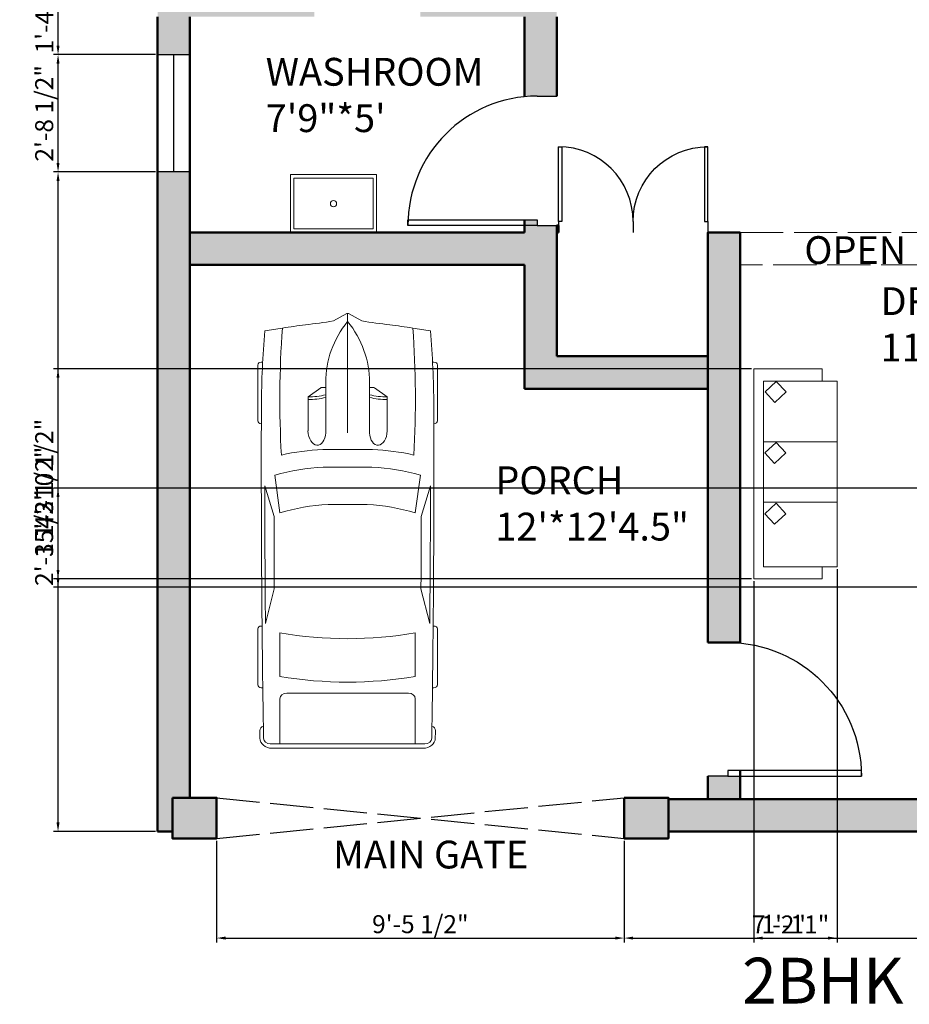
# Model space of a CAD drawing. Units: inches. Extents: x 876 to 1414, y 2665 to 3216.
# Tile 1 of 4: x 876 to 1124, y 2665 to 2939. Entities that reach past the tile are written whole.
import ezdxf

# ---------------------------------------------------------------- set-up
doc = ezdxf.new("R2010")
doc.units = ezdxf.units.IN
doc.linetypes.add('ACAD_ISO02W100', pattern=[15, 12, -3])
for name, color, linetype, lineweight in [('A-ANNO-DIMS', 2, 'Continuous', 18), ('A-ANNO-TEXT', 7, 'Continuous', 25), ('A-AREA-IDEN', 7, 'Continuous', 25), ('A-DOOR-GATE', 52, 'ACAD_ISO02W100', 25), ('A-FLOR-FIXT', 9, 'Continuous', 18), ('A-OPEN-OVHD', 210, 'ACAD_ISO02W100', 18), ('A-WALL-PATT', 252, 'Continuous', 13), ('CAR', 150, 'Continuous', 18), ('DOOR', 52, 'Continuous', 25), ('FUR', 8, 'Continuous', 18), ('WALL', 7, 'Continuous', 50), ('WIND', 130, 'Continuous', 25)]:
    doc.layers.add(name, color=color, linetype=linetype, lineweight=lineweight)
doc.styles.get("Standard").update_dxf_attribs({"font": 'arial.ttf'})
doc.dimstyles.new('ISO-25', dxfattribs={"dimtxt": 5, "dimasz": 2.5, "dimexe": 1.25, "dimexo": 0.625, "dimtad": 1, "dimdec": 0, "dimlunit": 4, "dimtxsty": 'Standard', "dimcen": 2.5, "dimadec": 0, "dimazin": 0, "dimtfac": 1, "dimtdec": 0, "dimtmove": 0, "dimatfit": 3, "dimfxl": 1, "dimarcsym": 0})

# ---------------------------------------------------------------- blocks, each defined once
blk = doc.blocks.new('*U2')
for p, q in [((0, 0), (0, -6)), ((40, 0), (40, -6))]:
    blk.add_line(p, q)
blk.add_lwpolyline([(0, 0), (0, 40), (1.75, 40), (1.75, 0)], close=True)
blk.add_arc((0, 0), 40, 0, 90)
blk = doc.blocks.new('*U4')
for p, q in [((46.55, 38.89), (22.35, 38.89)), ((136.7, 38.89), (160.9, 38.89)), ((21.1, 37.41), (21.1, 36.83)), ((47.8, 37.39), (47.8, 37.41)), ((87.99, 31.87), (74.76, 35.92)), ((134.31, 35.6), (119.29, 31.78)), ((135.45, 37.07), (135.45, 37.41)), ((162.15, 37.41), (162.15, 36.77)), ((70.03, 31.54), (86.41, 29.35)), ((186.47, -33.5), (186.47, 33.5)), ((188.4, -32.76), (188.4, 32.76)), ((138.42, 29.35), (157.25, 29.35)), ((164.52, 26.39), (164.52, -26.39)), ((186.47, 29.35), (167.01, 29.35)), ((32.27, 11.63), (36.13, 17.17)), ((36.13, 17.17), (50.94, 17.17)), ((29.77, 9.51), (51.68, 9.51)), ((32.12, 9.51), (32.12, 11.15)), ((58.92, -10.77), (58.92, 10.77)), ((66.55, -10.53), (66.55, 10.53)), ((186.47, -10.53), (186.47, 10.53)), ((3.27, 6.13), (0.1, 0.41)), ((82.74, 8.5), (82.74, -8.5)), ((0, 0), (51.68, 0)), ((0.1, -0.41), (3.27, -6.13)), ((29.77, -9.51), (51.68, -9.51)), ((32.12, -9.51), (32.12, -11.15)), ((32.27, -11.63), (36.13, -17.17)), ((36.13, -17.17), (50.94, -17.17)), ((86.41, -29.35), (70.03, -31.54)), ((157.25, -29.35), (138.42, -29.35)), ((167.01, -29.35), (186.47, -29.35)), ((87.99, -31.87), (74.76, -35.92)), ((134.31, -35.6), (119.29, -31.78)), ((21.1, -37.41), (21.1, -36.83)), ((47.8, -37.39), (47.8, -37.41)), ((135.45, -37.07), (135.45, -37.41)), ((162.15, -37.41), (162.15, -36.77)), ((46.55, -38.89), (22.35, -38.89)), ((136.7, -38.89), (160.9, -38.89))]:
    blk.add_line(p, q)
for centre, major_axis, ratio, start_param, end_param in [((22.35, 37.41), (0, -1.48), 0.842304, 3.141593, 4.712389), ((46.55, 37.41), (0, 1.48), 0.842304, -1.570796, 0), ((136.7, 37.41), (0, -1.48), 0.842304, 3.141593, 4.712389), ((160.9, 37.41), (0, 1.48), 0.842304, -1.570796, 0), ((266.03, -27.52), (0, 313.31), 0.842304, 1.367076, 1.39176), ((41.19, -490.86), (0, 528.23), 0.842304, 0.00281, 0.075598), ((64.48, -10555.62), (0, 10593.03), 0.842304, -0.013397, 0.002797), ((64.48, -10555.62), (0, -10591.55), 0.842304, 3.133765, 3.140441), ((180.63, 35.84), (0, 2.22), 0.842304, -0.013017, 1.249894), ((64.48, -10556.36), (0, 10595.31), 0.842304, -0.013397, -0.013017), ((183.98, 33.5), (0, -2.96), 0.842304, 1.570796, 3.128196), ((183.98, 32.76), (0, -5.25), 0.842304, 1.570796, 3.128196), ((135.29, 5.39), (0, 81.77), 0.842304, 1.245306, 1.50788), ((95.79, -3666.35), (0, -3698.24), 0.842304, 3.134049, 3.144098), ((259.18, -27.52), (0, -305.3), 0.842304, 4.528606, 4.561838), ((37.47, -593.96), (0, -623.33), 0.842304, 3.096046, 3.200911), ((134.4, 5.39), (0, -89.78), 0.842304, 4.449482, 4.652344), ((149.6, 2.8), (0, -79.58), 0.842304, 4.372215, 4.640744), ((17.08, 0), (0, 147.02), 0.842304, 4.511394, 4.913384), ((35.91, 0), (0, 147.02), 0.842304, 4.511394, 4.913384), ((167.01, 26.39), (0, 2.96), 0.842304, 0, 1.570796), ((-204.49, 52.4), (0, -250.96), 0.842304, 1.385369, 1.434372), ((13.04, 17.01), (0, 27.42), 0.842304, 4.435146, 4.718221), ((14.2, 17.01), (0, 27.42), 0.842304, 4.435146, 4.718221), ((50.79, 13.34), (6.34, -0.36), 0.603834, -1.395552, 1.581315), ((29.77, -46.66), (0, 56.17), 0.842304, 0, 0.590319), ((32.75, 11.15), (0, 0.74), 0.842304, 0.879714, 1.570796), ((0.62, 0), (0, -0.74), 0.842304, 4.131459, 5.293319), ((29.77, 46.66), (0, 56.17), 0.842304, 2.551274, 3.141593), ((-204.49, -52.4), (0, 250.96), 0.842304, -1.434372, -1.385369), ((149.6, -2.8), (0, -79.58), 0.842304, -1.499151, -1.230623), ((32.75, -11.15), (0, -0.74), 0.842304, 4.712389, 5.403472), ((13.04, -17.01), (0, -27.42), 0.842304, 1.564964, 1.848039), ((14.2, -17.01), (0, -27.42), 0.842304, 1.564964, 1.848039), ((134.4, -5.39), (0, -89.78), 0.842304, -1.510751, -1.307889), ((135.29, -5.39), (0, -81.77), 0.842304, -1.50788, -1.245306), ((259.18, 27.52), (0, 305.3), 0.842304, 1.721348, 1.754579), ((266.03, 27.52), (0, 313.31), 0.842304, 1.749832, 1.774517), ((37.47, 593.96), (0, -623.33), 0.842304, -0.059319, 0.045547), ((167.01, -26.39), (0, -2.96), 0.842304, 4.712389, 6.283185), ((95.79, 3666.35), (0, -3698.24), 0.842304, -0.002505, 0.007544), ((183.98, -33.5), (0, 2.96), 0.842304, 3.15499, 4.712389), ((183.98, -32.76), (0, -5.25), 0.842304, 0.013397, 1.570796), ((41.19, 490.86), (0, -528.23), 0.842304, -0.075598, -0.00281), ((22.35, -37.41), (0, 1.48), 0.842304, 1.570796, 3.141593), ((64.48, 10555.62), (0, 10593.03), 0.842304, 3.138796, 3.15499), ((46.55, -37.41), (0, -1.48), 0.842304, 0, 1.570796), ((64.48, 10555.62), (0, -10591.55), 0.842304, 0.001152, 0.007828), ((136.7, -37.41), (0, -1.48), 0.842304, -1.570796, 0), ((160.9, -37.41), (0, 1.48), 0.842304, 3.141593, 4.712389), ((180.63, -35.84), (0, -2.22), 0.842304, -1.249894, 0.013017), ((64.48, 10556.36), (0, 10595.31), 0.842304, 3.15461, 3.15499)]:
    blk.add_ellipse(centre, major_axis=major_axis, ratio=ratio, start_param=start_param, end_param=end_param)
at = {"extrusion": (0, 0, -1)}
blk.add_ellipse((50.79, -13.34), major_axis=(6.34, 0.36), ratio=0.603834, start_param=-1.395552, end_param=1.581315, dxfattribs=at)
blk = doc.blocks.new('*D31')
at = {"layer": 'A-ANNO-DIMS', "color": 0, "lineweight": -2, "transparency": 16777216}
for p, q in [((1128.58, 2808.89), (885.57, 2808.89)), ((886.82, 2783.86), (886.82, 2806.39)), ((1128.58, 2781.36), (885.57, 2781.36))]:
    blk.add_line(p, q, dxfattribs=at)
at = {"layer": 'A-ANNO-DIMS', "color": 0, "lineweight": 100, "transparency": 16777216}
for points in [[(886.4, 2806.39), (887.23, 2806.39), (886.82, 2808.89)], [(886.4, 2783.86), (887.23, 2783.86), (886.82, 2781.36)]]:
    blk.add_solid(points, dxfattribs=at)
at = {"layer": 'Defpoints', "color": 0, "lineweight": 100, "transparency": 16777216}
for p in [(886.82, 2808.89), (1129.2, 2808.89), (1129.2, 2781.36)]:
    blk.add_point(p, dxfattribs=at)
at = {"layer": 'A-ANNO-DIMS', "color": 0, "transparency": 16777216, "insert": (883.6, 2795.13), "char_height": 5, "attachment_point": 5, "rotation": 90}
blk.add_mtext('2\'-3 1/2"', dxfattribs=at)
blk = doc.blocks.new('*D32')
at = {"layer": 'A-ANNO-DIMS', "color": 0, "lineweight": -2, "transparency": 16777216}
for p, q in [((1079.71, 2842.08), (885.57, 2842.08)), ((886.82, 2786.17), (886.82, 2839.58)), ((1079.71, 2783.67), (885.57, 2783.67))]:
    blk.add_line(p, q, dxfattribs=at)
at = {"layer": 'A-ANNO-DIMS', "color": 0, "lineweight": 100, "transparency": 16777216}
for points in [[(886.4, 2839.58), (887.23, 2839.58), (886.82, 2842.08)], [(886.4, 2786.17), (887.23, 2786.17), (886.82, 2783.67)]]:
    blk.add_solid(points, dxfattribs=at)
at = {"layer": 'Defpoints', "color": 0, "lineweight": 100, "transparency": 16777216}
for p in [(886.82, 2842.08), (1080.33, 2842.08), (1080.33, 2783.67)]:
    blk.add_point(p, dxfattribs=at)
at = {"layer": 'A-ANNO-DIMS', "color": 0, "transparency": 16777216, "insert": (883.61, 2812.87), "char_height": 5, "attachment_point": 5, "rotation": 90}
blk.add_mtext('4\'-10 1/2"', dxfattribs=at)
blk = doc.blocks.new('*D33')
at = {"layer": 'A-ANNO-DIMS', "color": 0, "lineweight": -2, "transparency": 16777216}
for p, q in [((1103.5, 2786.39), (1103.5, 2682.56)), ((1080.33, 2783.04), (1080.33, 2682.56)), ((1082.83, 2683.81), (1101, 2683.81))]:
    blk.add_line(p, q, dxfattribs=at)
at = {"layer": 'A-ANNO-DIMS', "color": 0, "lineweight": 100, "transparency": 16777216}
for points in [[(1082.83, 2684.22), (1082.83, 2683.39), (1080.33, 2683.81)], [(1101, 2684.22), (1101, 2683.39), (1103.5, 2683.81)]]:
    blk.add_solid(points, dxfattribs=at)
at = {"layer": 'Defpoints', "color": 0, "lineweight": 100, "transparency": 16777216}
for p in [(1103.5, 2787.02), (1080.33, 2783.67), (1103.5, 2683.81)]:
    blk.add_point(p, dxfattribs=at)
at = {"layer": 'A-ANNO-DIMS', "color": 0, "transparency": 16777216, "insert": (1091.91, 2686.94), "char_height": 5, "attachment_point": 5}
blk.add_mtext('1\'-11"', dxfattribs=at)
blk = doc.blocks.new('*D41')
at = {"layer": 'A-ANNO-DIMS', "color": 0, "lineweight": -2, "transparency": 16777216}
for p, q in [((930.9, 2710.88), (930.9, 2682.56)), ((1044.28, 2710.88), (1044.28, 2682.56)), ((933.4, 2683.81), (1041.78, 2683.81))]:
    blk.add_line(p, q, dxfattribs=at)
at = {"layer": 'A-ANNO-DIMS', "color": 0, "lineweight": 100, "transparency": 16777216}
for points in [[(933.4, 2684.22), (933.4, 2683.39), (930.9, 2683.81)], [(1041.78, 2684.22), (1041.78, 2683.39), (1044.28, 2683.81)]]:
    blk.add_solid(points, dxfattribs=at)
at = {"layer": 'Defpoints', "color": 0, "lineweight": 100, "transparency": 16777216}
for p in [(930.9, 2711.51), (1044.28, 2711.51), (1044.28, 2683.81)]:
    blk.add_point(p, dxfattribs=at)
at = {"layer": 'A-ANNO-DIMS', "color": 0, "transparency": 16777216, "insert": (987.59, 2687.02), "char_height": 5, "attachment_point": 5}
blk.add_mtext('9\'-5 1/2"', dxfattribs=at)
blk = doc.blocks.new('*D42')
at = {"layer": 'A-ANNO-DIMS', "color": 0, "lineweight": -2, "transparency": 16777216}
for p, q in [((1130.38, 2712.82), (1130.38, 2682.56)), ((1044.28, 2710.88), (1044.28, 2682.56)), ((1046.78, 2683.81), (1127.88, 2683.81))]:
    blk.add_line(p, q, dxfattribs=at)
at = {"layer": 'A-ANNO-DIMS', "color": 0, "lineweight": 100, "transparency": 16777216}
for points in [[(1046.78, 2684.22), (1046.78, 2683.39), (1044.28, 2683.81)], [(1127.88, 2684.22), (1127.88, 2683.39), (1130.38, 2683.81)]]:
    blk.add_solid(points, dxfattribs=at)
at = {"layer": 'Defpoints', "color": 0, "lineweight": 100, "transparency": 16777216}
for p in [(1130.38, 2713.44), (1044.28, 2711.51), (1130.38, 2683.81)]:
    blk.add_point(p, dxfattribs=at)
at = {"layer": 'A-ANNO-DIMS', "color": 0, "transparency": 16777216, "insert": (1087.33, 2686.94), "char_height": 5, "attachment_point": 5}
blk.add_mtext('7\'-2"', dxfattribs=at)
blk = doc.blocks.new('*D51')
at = {"layer": 'A-ANNO-DIMS', "color": 0, "lineweight": -2, "transparency": 16777216}
for p, q in [((913.89, 2945.19), (885.57, 2945.19)), ((886.82, 2931.91), (886.82, 2942.69)), ((913.89, 2929.41), (885.57, 2929.41))]:
    blk.add_line(p, q, dxfattribs=at)
at = {"layer": 'A-ANNO-DIMS', "color": 0, "lineweight": 100, "transparency": 16777216}
for points in [[(886.4, 2942.69), (887.23, 2942.69), (886.82, 2945.19)], [(886.4, 2931.91), (887.23, 2931.91), (886.82, 2929.41)]]:
    blk.add_solid(points, dxfattribs=at)
at = {"layer": 'Defpoints', "color": 0, "lineweight": 100, "transparency": 16777216}
for p in [(886.82, 2945.19), (914.52, 2945.19), (914.52, 2929.41)]:
    blk.add_point(p, dxfattribs=at)
at = {"layer": 'A-ANNO-DIMS', "color": 0, "transparency": 16777216, "insert": (883.68, 2937.3), "char_height": 5, "attachment_point": 5, "rotation": 90}
blk.add_mtext('1\'-4"', dxfattribs=at)
blk = doc.blocks.new('*D52')
at = {"layer": 'A-ANNO-DIMS', "color": 0, "lineweight": -2, "transparency": 16777216}
for p, q in [((913.89, 2929.41), (885.57, 2929.41)), ((886.82, 2899.3), (886.82, 2926.91)), ((913.89, 2896.8), (885.57, 2896.8))]:
    blk.add_line(p, q, dxfattribs=at)
at = {"layer": 'A-ANNO-DIMS', "color": 0, "lineweight": 100, "transparency": 16777216}
for points in [[(886.4, 2926.91), (887.23, 2926.91), (886.82, 2929.41)], [(886.4, 2899.3), (887.23, 2899.3), (886.82, 2896.8)]]:
    blk.add_solid(points, dxfattribs=at)
at = {"layer": 'Defpoints', "color": 0, "lineweight": 100, "transparency": 16777216}
for p in [(886.82, 2929.41), (914.52, 2929.41), (914.52, 2896.8)]:
    blk.add_point(p, dxfattribs=at)
at = {"layer": 'A-ANNO-DIMS', "color": 0, "transparency": 16777216, "insert": (883.61, 2913.1), "char_height": 5, "attachment_point": 5, "rotation": 90}
blk.add_mtext('2\'-8 1/2"', dxfattribs=at)
blk = doc.blocks.new('*D53')
at = {"layer": 'A-ANNO-DIMS', "color": 0, "lineweight": -2, "transparency": 16777216}
for p, q in [((913.89, 2896.8), (885.57, 2896.8)), ((886.82, 2715.94), (886.82, 2894.3)), ((913.89, 2713.44), (885.57, 2713.44))]:
    blk.add_line(p, q, dxfattribs=at)
at = {"layer": 'A-ANNO-DIMS', "color": 0, "lineweight": 100, "transparency": 16777216}
for points in [[(886.4, 2894.3), (887.23, 2894.3), (886.82, 2896.8)], [(886.4, 2715.94), (887.23, 2715.94), (886.82, 2713.44)]]:
    blk.add_solid(points, dxfattribs=at)
at = {"layer": 'Defpoints', "color": 0, "lineweight": 100, "transparency": 16777216}
for p in [(886.82, 2896.8), (914.52, 2896.8), (914.52, 2713.44)]:
    blk.add_point(p, dxfattribs=at)
at = {"layer": 'A-ANNO-DIMS', "color": 0, "transparency": 16777216, "insert": (883.6, 2805.12), "char_height": 5, "attachment_point": 5, "rotation": 90}
blk.add_mtext('15\'-3 1/2"', dxfattribs=at)

msp = doc.modelspace()

# ---------------------------------------------------------------- hatches: boundary and pattern name
at = {"layer": 'A-WALL-PATT'}
h = msp.add_hatch(color=256, dxfattribs=at)
h.dxf.hatch_style = 1
h.paths.add_polyline_path([(966.14, 3166.44), (914.52, 3166.44), (914.52, 3077.43), (923.52, 3077.43), (923.52, 3157.44), (966.14, 3157.44)])
h.paths.add_polyline_path([(1117.41, 3166.44), (1072.02, 3166.44), (1025.39, 3166.44), (1025.39, 3157.44), (1067.52, 3157.44), (1067.52, 3050.33), (1068, 3050.33), (1068, 3010.33), (1068, 3004.44), (1072.02, 3004.44), (1076.39, 3004.44), (1076.39, 3010.44), (1076.39, 3013.44), (1072.02, 3013.44), (1072.02, 3157.44), (1090.31, 3157.44), (1117.41, 3157.44)])
h.paths.add_polyline_path([(1257.93, 3166.44), (1225.02, 3166.44), (1176.66, 3166.44), (1176.66, 3157.44), (1216.02, 3157.44), (1216.02, 3013.44), (1116.28, 3013.44, -0.01877), (1116.39, 3010.44), (1116.39, 3004.44), (1225.02, 3004.44), (1225.02, 3014.27), (1225.02, 3110.94), (1249.02, 3110.94), (1251.21, 3110.94), (1251.21, 3115.44), (1225.02, 3115.44), (1225.02, 3157.44), (1257.93, 3157.44)])
h.paths.add_polyline_path([(1361.52, 3166.44), (1317.18, 3166.44), (1317.18, 3157.44), (1330.83, 3157.44), (1352.52, 3157.44), (1352.52, 3115.44), (1288.77, 3115.44), (1288.77, 3110.94), (1352.52, 3110.94), (1352.52, 3103.98), (1361.52, 3103.98), (1361.52, 3115.44)])
h.paths.add_polyline_path([(1028, 3010.33, -0.01947), (1028.12, 3013.44), (985.91, 3013.44), (985.91, 3004.44), (1028, 3004.44)])
h.paths.add_polyline_path([(953.71, 3013.44), (923.52, 3013.44), (923.52, 3018.18), (914.52, 3018.18), (914.52, 3004.44), (923.52, 3004.44), (953.71, 3004.44)])
h.paths.add_polyline_path([(958.09, 2944.44), (923.52, 2944.44), (923.52, 2945.19), (914.52, 2945.19), (914.52, 2939.94), (914.52, 2929.41), (923.52, 2929.41), (923.52, 2939.94), (958.09, 2939.94)])
h.paths.add_polyline_path([(1025.52, 3004.44), (1016.52, 3004.44), (1016.52, 2944.44), (987.59, 2944.44), (987.59, 2939.94), (1016.52, 2939.94), (1016.52, 2917.71, -0.025042), (1020.12, 2917.89), (1025.52, 2917.89), (1025.52, 2939.94)])
h.paths.add_polyline_path([(923.52, 2870.94), (923.52, 2879.94), (923.52, 2896.8), (914.52, 2896.8), (914.52, 2870.94), (914.52, 2713.44), (918.61, 2713.44), (918.61, 2722.81), (923.52, 2722.81)])
h.paths.add_polyline_path([(930.9, 2722.81), (918.61, 2722.81), (918.61, 2711.51), (930.9, 2711.51)])
h.paths.add_polyline_path([(1056.58, 2722.81), (1044.28, 2722.81), (1044.28, 2711.51), (1056.58, 2711.51)])
h.paths.add_polyline_path([(1130.38, 2722.44), (1076.52, 2722.44), (1067.52, 2722.44), (1056.58, 2722.44), (1056.58, 2713.44), (1076.52, 2713.44), (1130.38, 2713.44)])
h.paths.add_polyline_path([(1213.02, 2879.94), (1142.76, 2879.94), (1142.76, 2870.94), (1208.52, 2870.94), (1208.52, 2722.44), (1213.02, 2722.44)])
h.paths.add_polyline_path([(1219.02, 2822.94), (1213.02, 2822.94), (1213.02, 2818.44), (1219.02, 2818.44)])
h.paths.add_polyline_path([(1352.52, 2822.94), (1259.02, 2822.94), (1259.02, 2818.44), (1352.52, 2818.44)])
h.paths.add_polyline_path([(1274.52, 2848.67), (1270.02, 2848.67), (1270.02, 2822.94), (1274.52, 2822.94)])
h.paths.add_polyline_path([(1352.52, 2887.44), (1270.02, 2887.44), (1270.02, 2880.56), (1274.52, 2880.56), (1274.52, 2882.94), (1352.52, 2882.94)])
h.paths.add_polyline_path([(1361.52, 2915.4), (1352.52, 2915.4), (1352.52, 2872.66), (1361.52, 2872.66)])
h.paths.add_polyline_path([(1361.52, 2840.05), (1352.52, 2840.05), (1352.52, 2722.44), (1319.37, 2722.44), (1319.37, 2713.44), (1349.52, 2713.44), (1361.52, 2713.44)])
h.paths.add_polyline_path([(1260.12, 2722.44), (1225.02, 2722.44), (1213.02, 2722.44), (1208.52, 2722.44), (1189.62, 2722.44), (1189.62, 2713.44), (1213.02, 2713.44), (1260.12, 2713.44)])
h.paths.add_polyline_path([(1361.52, 3004.44), (1361.52, 3044.73), (1352.52, 3044.73), (1352.52, 3013.44), (1352.52, 2974.65), (1361.52, 2974.65)])
h.paths.add_polyline_path([(1352.52, 3013.44), (1288.77, 3013.44), (1288.77, 3004.44), (1352.52, 3004.44)])
h.paths.add_polyline_path([(1067.52, 2845.54), (1025.52, 2845.54), (1025.52, 2870.94), (1025.52, 2881.89), (1020.12, 2881.89), (1016.52, 2881.89), (1016.52, 2879.94), (923.52, 2879.94), (923.52, 2870.94), (1016.52, 2870.94), (1016.52, 2845.54), (1016.52, 2836.54), (1025.52, 2836.54), (1067.52, 2836.54)])
h.paths.add_polyline_path([(1076.52, 2728.79), (1073.09, 2728.79), (1067.52, 2728.79), (1067.52, 2722.44), (1076.52, 2722.44)])
h.paths.add_polyline_path([(1091.93, 2866.85), (1126.41, 2866.85), (1126.41, 2882.79), (1091.93, 2882.79)], flags=9)
h.paths.add_polyline_path([(1112.49, 2839.74), (1177.4, 2839.74), (1177.4, 2868.59), (1112.49, 2868.59)], flags=9)
h.paths.add_polyline_path([(1005.34, 2789.94), (1060.41, 2789.94), (1060.41, 2818.8), (1005.34, 2818.8)], flags=9)
h = msp.add_hatch(color=256, dxfattribs=at)
h.dxf.hatch_style = 1
h.paths.add_polyline_path([(1020.12, 2883.47), (1016.52, 2883.47), (1016.52, 2881.89), (1020.12, 2881.89)])
h = msp.add_hatch(color=256, dxfattribs=at)
h.dxf.hatch_style = 1
h.paths.add_polyline_path([(1076.52, 2879.94), (1067.52, 2879.94), (1067.52, 2765.95), (1076.52, 2765.95)])

# ---------------------------------------------------------------- linework, layer by layer
at = {"layer": 'A-DOOR-GATE'}
for p, q in [((930.9, 2711.51), (1044.28, 2722.81)), ((930.9, 2722.81), (1044.28, 2711.51))]:
    msp.add_line(p, q, dxfattribs=at)
at = {"layer": 'A-FLOR-FIXT'}
for points in [[(975.44, 2879.94), (951.44, 2879.94), (951.44, 2896.06), (975.44, 2896.06)], [(974.44, 2880.94), (952.44, 2880.94), (952.44, 2895.06), (974.44, 2895.06)]]:
    msp.add_lwpolyline(points, close=True, dxfattribs=at)
msp.add_circle((963.44, 2888), 0.871, dxfattribs=at)
at = {"layer": 'A-OPEN-OVHD'}
msp.add_lwpolyline([(1076.52, 2879.94), (1142.76, 2879.94), (1142.76, 2870.94), (1076.52, 2870.94)], close=True, dxfattribs=at)
at = {"layer": 'FUR'}
for p, q in [((1099.32, 2842.08), (1080.33, 2842.08)), ((1080.33, 2842.08), (1080.33, 2783.67)), ((1099.32, 2838.61), (1099.32, 2842.08)), ((1083.08, 2821.79), (1103.5, 2821.79)), ((1083.08, 2805.03), (1103.5, 2805.03)), ((1099.32, 2783.67), (1099.32, 2787.02)), ((1080.33, 2783.67), (1099.32, 2783.67))]:
    msp.add_line(p, q, dxfattribs=at)
for points in [[(1083.08, 2787.02), (1103.5, 2787.02), (1103.5, 2838.61), (1083.08, 2838.61)], [(1089.31, 2835.64), (1086.17, 2832.73), (1083.47, 2835.64), (1086.6, 2838.56)], [(1089.24, 2818.67), (1086.1, 2815.75), (1083.4, 2818.67), (1086.53, 2821.58)], [(1089.24, 2801.78), (1086.1, 2798.87), (1083.4, 2801.78), (1086.53, 2804.69)]]:
    msp.add_lwpolyline(points, close=True, dxfattribs=at)
at = {"layer": 'WALL'}
for p, q in [((914.52, 2939.94), (914.52, 2870.94)), ((923.52, 2939.94), (923.52, 2879.94)), ((1016.52, 2917.71), (1016.52, 2939.94)), ((1025.52, 2917.89), (1025.52, 2939.94)), ((1016.52, 2879.94), (1016.52, 2883.47)), ((923.52, 2879.94), (1016.52, 2879.94)), ((923.52, 2879.94), (923.52, 2870.94)), ((1025.52, 2870.94), (1025.52, 2881.89)), ((1067.52, 2879.94), (1067.52, 2840.71)), ((1076.52, 2879.94), (1067.52, 2879.94)), ((1076.52, 2870.94), (1076.52, 2879.94)), ((914.52, 2870.94), (914.52, 2713.44)), ((923.52, 2870.94), (1016.52, 2870.94)), ((923.52, 2870.94), (923.52, 2722.81)), ((1016.52, 2870.94), (1016.52, 2845.54)), ((1025.52, 2870.94), (1025.52, 2845.54)), ((1076.52, 2870.94), (1076.52, 2840.71)), ((1016.52, 2845.54), (1016.52, 2836.54)), ((1025.52, 2845.54), (1067.52, 2845.54)), ((1067.52, 2765.95), (1067.52, 2845.54)), ((1076.52, 2765.8), (1076.52, 2845.54)), ((1016.52, 2836.54), (1025.52, 2836.54)), ((1025.52, 2836.54), (1067.52, 2836.54)), ((1076.52, 2722.44), (1076.52, 2730.41)), ((1067.52, 2722.44), (1067.52, 2728.79)), ((1056.58, 2722.44), (1067.52, 2722.44)), ((1067.52, 2722.44), (1076.52, 2722.44)), ((1076.52, 2722.44), (1208.52, 2722.44)), ((914.52, 2713.44), (918.61, 2713.44)), ((1056.58, 2713.44), (1076.52, 2713.44)), ((1076.52, 2713.44), (1213.02, 2713.44))]:
    msp.add_line(p, q, dxfattribs=at)
for points in [[(1026.01, 2879.94), (1025.52, 2879.94), (1025.52, 2881.89), (1026.01, 2881.89)], [(1067.52, 2765.95), (1076.52, 2765.95), (1076.52, 2879.94), (1067.52, 2879.94)], [(918.61, 2722.81), (930.9, 2722.81), (930.9, 2711.51), (918.61, 2711.51)], [(1044.28, 2722.81), (1056.58, 2722.81), (1056.58, 2711.51), (1044.28, 2711.51)]]:
    msp.add_lwpolyline(points, close=True, dxfattribs=at)
at = {"layer": 'WIND'}
msp.add_line((919.02, 2896.8), (919.02, 2929.41), dxfattribs=at)
msp.add_lwpolyline([(914.52, 2929.41), (923.52, 2929.41), (923.52, 2896.8), (914.52, 2896.8)], close=True, dxfattribs=at)

# ---------------------------------------------------------------- block references
at = {"layer": 'CAR', "xscale": 0.6417008015974152, "yscale": 0.6417008015974152, "zscale": 0.6417008015974152, "rotation": 270}
msp.add_blockref('*U4', (967.36, 2857.47), dxfattribs=at)
at = {"layer": 'DOOR'}
for p, xscale, yscale, zscale, rotation in [((1020.12, 2881.89), 0.9000758785505945, 0.9000758785505945, 0.9000758785505945, 90), ((1073.09, 2728.79), -0.9291160392037722, 0.9291160392037722, 0.9291160392037722, 270)]:
    msp.add_blockref('*U2', p, dxfattribs=dict(at, xscale=xscale, yscale=yscale, zscale=zscale, rotation=rotation))
at = {"layer": 'DOOR', "yscale": 0.5188432195801443, "zscale": 0.5188432195801443}
for p, xscale in [((1026.01, 2883.05), 0.5188432195801443), ((1067.52, 2883.05), -0.5188432195801443)]:
    msp.add_blockref('*U2', p, dxfattribs=dict(at, xscale=xscale))

# ---------------------------------------------------------------- texts
at = {"layer": 'A-ANNO-TEXT', "attachment_point": 1}
for s, width, gutter_width, insert, char_height in [('OPEN', 254.6465, 38.66, (1094.39, 2878.94), 7.733), ('MAIN GATE', 254.6465, 38.66, (963.33, 2710.89), 7.733), ('2BHK HOUSE PLAN', 418.7884, 63.58, (1077.09, 2678.33), 12.7168)]:
    msp.add_mtext_dynamic_manual_height_columns(s, width=width, gutter_width=gutter_width, heights=[0], dxfattribs=dict(at, insert=insert, char_height=char_height))
at = {"layer": 'A-AREA-IDEN', "attachment_point": 1}
for s, insert, char_height in [('WASHROOM\\P7\'9"*5\'', (944.58, 2928.51), 7.733), ('DRG ROOM\\P11\'9"*12\'4.5"', (1115.59, 2864.75), 7.7325), ('PORCH\\P12\'*12\'4.5"', (1008.45, 2814.95), 7.7325)]:
    msp.add_mtext_dynamic_manual_height_columns(s, width=254.6465, gutter_width=38.66, heights=[0], dxfattribs=dict(at, insert=insert, char_height=char_height))

# ---------------------------------------------------------------- dimensions: what is measured, and where the dimension line sits
at = {"layer": 'A-ANNO-DIMS'}
for base, p1, p2, picture, middle in [((886.82, 2945.19), (914.52, 2929.41), (914.52, 2945.19), '*D51', (883.68, 2937.3)), ((886.82, 2929.41), (914.52, 2896.8), (914.52, 2929.41), '*D52', (883.61, 2913.1)), ((886.82, 2896.8), (914.52, 2713.44), (914.52, 2896.8), '*D53', (883.6, 2805.12)), ((886.82, 2842.08), (1080.33, 2783.67), (1080.33, 2842.08), '*D32', (883.61, 2812.87)), ((886.82, 2808.89), (1129.2, 2781.36), (1129.2, 2808.89), '*D31', (883.6, 2795.13))]:
    dim = msp.add_linear_dim(base=base, p1=p1, p2=p2, angle=90, dimstyle='ISO-25', override={"dimdec": 1, "dimlfac": 1, "dimrnd": 0, "dimzin": 1, "dimdsep": 46, "dimlunit": 4, "dimfrac": 2}, dxfattribs=at)
    dim.commit()
    dim.dimension.update_dxf_attribs({"geometry": picture, "text_midpoint": middle})
for base, p1, p2, picture, middle in [((1103.5, 2683.81), (1080.33, 2783.67), (1103.5, 2787.02), '*D33', (1091.91, 2686.94)), ((1130.38, 2683.81), (1044.28, 2711.51), (1130.38, 2713.44), '*D42', (1087.33, 2686.94)), ((1044.28, 2683.81), (930.9, 2711.51), (1044.28, 2711.51), '*D41', (987.59, 2687.02))]:
    dim = msp.add_linear_dim(base=base, p1=p1, p2=p2, dimstyle='ISO-25', override={"dimdec": 1, "dimlfac": 1, "dimrnd": 0, "dimzin": 1, "dimdsep": 46, "dimlunit": 4, "dimfrac": 2}, dxfattribs=at)
    dim.commit()
    dim.dimension.update_dxf_attribs({"geometry": picture, "text_midpoint": middle})

doc.saveas('drawing.dxf')
